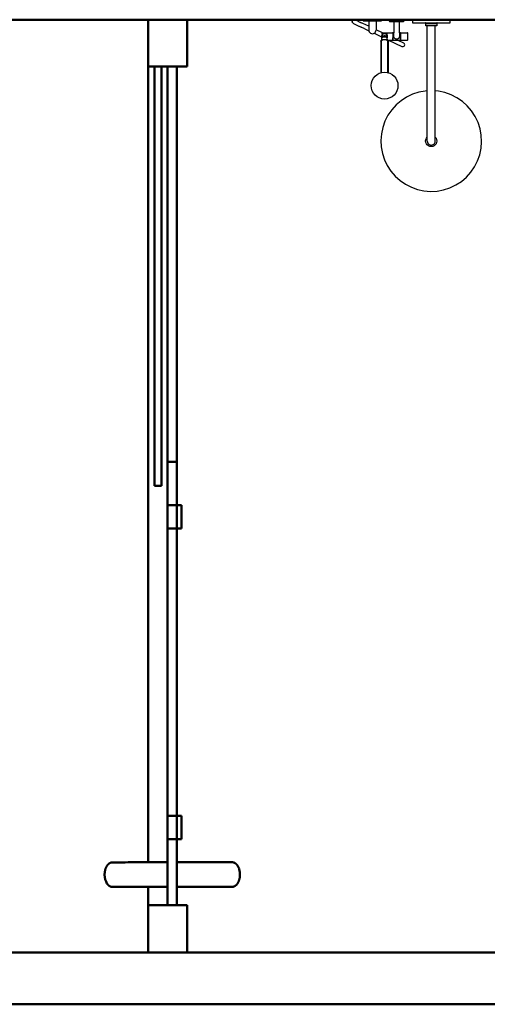
# Model space of a CAD drawing. Units: inches. Extents: x 64 to 1167, y 117 to 939.
# Tile 18 of 56: x 248 to 284, y 781 to 857. Entities that reach past the tile are written whole.
import ezdxf

# ---------------------------------------------------------------- set-up
doc = ezdxf.new("R2010")
doc.units = ezdxf.units.IN
doc.header["$MEASUREMENT"] = 0
doc.layers.add('A-FLOR-FIXT', color=8, linetype='Continuous', lineweight=18)
doc.layers.add('A-WALL', color=7, linetype='Continuous', lineweight=50)
doc.layers.add('Edges', color=7, linetype='Continuous')

# ---------------------------------------------------------------- blocks, each defined once
blk = doc.blocks.new('Handheld Shower set pl')
at = {"layer": 'Edges'}
for p, q in [((254.9, 328.7), (274.2, 319.6)), ((262, 340.8), (280.2, 332.2)), ((274.2, 319.6), (276.7, 318.4)), ((279.6, 317), (276.7, 318.4)), ((279.6, 317), (281.6, 316)), ((287.6, 328.7), (280.2, 332.2)), ((280.2, 332.2), (282.7, 331)), ((294.8, 309.8), (281.6, 316)), ((308.3, 318.9), (287.6, 328.7)), ((352.8, 340.8), (289.3, 340.8)), ((289.3, 340.8), (289.3, 337.7)), ((289.3, 337.7), (308.4, 337.7)), ((294.8, 309.8), (308.8, 303.2)), ((308.3, 318.9), (308.4, 318.8)), ((308.4, 337.7), (308.4, 318.8)), ((308.4, 337.7), (333.8, 337.7)), ((308.4, 318.8), (308.4, 305.9)), ((333.8, 337.7), (333.8, 306.8)), ((333.8, 337.7), (352.8, 337.7)), ((352.8, 340.8), (352.8, 337.7)), ((379.7, 340.5), (379.7, 336.5)), ((380.1, 340.7), (430.2, 340.7)), ((380.1, 336.2), (430.2, 336.2)), ((381.6, 335.3), (428.8, 335.3)), ((395.6, 335.3), (395.6, 296.4)), ((414.6, 296.4), (414.6, 335.3)), ((430.5, 340.5), (430.5, 336.5)), ((460.1, 340.8), (460.1, 330.7)), ((591.7, 340.8), (460.1, 340.8)), ((460.1, 330.7), (505.5, 330.7)), ((505.7, 330.7), (505.5, 330.7)), ((505.9, 330.6), (505.7, 330.7)), ((505.7, 330.7), (545.6, 330.7)), ((506.1, 330.5), (505.9, 330.6)), ((506.3, 330.4), (506.1, 330.5)), ((506.5, 330.3), (506.3, 330.4)), ((506.6, 330.1), (506.5, 330.3)), ((506.7, 329.9), (506.6, 330.1)), ((506.8, 329.7), (506.7, 329.9)), ((506.9, 329.5), (506.8, 329.7)), ((506.9, 329.3), (506.9, 329.5)), ((506.9, 329.1), (506.9, 329.3)), ((544.4, 329.1), (506.9, 329.1)), ((506.9, 320.4), (506.9, 328.9)), ((506.9, 328.9), (544.4, 328.9)), ((511.4, 320.4), (506.9, 320.4)), ((511.4, 94.2), (511.4, 320.4)), ((539.4, 320.4), (511.4, 320.4)), ((539.4, 94.2), (539.4, 320.4)), ((544.4, 320.4), (539.4, 320.4)), ((544.5, 329.5), (544.4, 329.3)), ((544.4, 329.3), (544.4, 329.1)), ((544.4, 328.9), (544.4, 320.4)), ((544.6, 329.9), (544.5, 329.7)), ((544.5, 329.7), (544.5, 329.5)), ((544.7, 330.1), (544.6, 329.9)), ((544.9, 330.3), (544.7, 330.1)), ((545, 330.4), (544.9, 330.3)), ((545.2, 330.5), (545, 330.4)), ((545.4, 330.6), (545.2, 330.5)), ((545.6, 330.7), (545.4, 330.6)), ((545.8, 330.7), (545.6, 330.7)), ((545.8, 330.7), (591.7, 330.7)), ((591.7, 330.7), (591.7, 340.8)), ((308.4, 305.9), (308.8, 303.2)), ((308.8, 303.2), (308.8, 302.6)), ((308.8, 302.6), (310.1, 299.6)), ((310.1, 299.6), (312.1, 296.9)), ((312.1, 296.9), (314.7, 294.9)), ((314.7, 294.9), (317.8, 293.7)), ((317.8, 293.7), (321.1, 293.2)), ((321.1, 293.2), (324.4, 293.7)), ((324.4, 293.7), (326.7, 294.6)), ((326.7, 294.6), (327.4, 294.9)), ((326.7, 294.6), (352.9, 282.2)), ((327.4, 294.9), (330.1, 296.9)), ((330.1, 296.9), (332.1, 299.6)), ((332.1, 299.6), (333.4, 302.6)), ((333.4, 302.6), (333.8, 305.9)), ((333.8, 306.8), (333.8, 305.9)), ((355.7, 296.4), (333.8, 306.8)), ((352.9, 285.6), (352.8, 284.3)), ((352.8, 284.3), (352.8, 283)), ((352.8, 283), (352.9, 282.2)), ((353.2, 286.9), (352.9, 285.6)), ((352.9, 282.2), (352.9, 281.8)), ((352.9, 281.8), (353.2, 280.5)), ((353.7, 288.1), (353.2, 286.9)), ((353.2, 280.5), (353.6, 279.7)), ((353.5, 296.4), (355.7, 296.4)), ((353.5, 296.4), (353.5, 293.2)), ((353.5, 293.2), (359.1, 293.2)), ((353.5, 274.2), (353.6, 278.1)), ((353.5, 271.2), (353.5, 274.2)), ((353.5, 274.2), (353.6, 274.2)), ((353.7, 285.5), (353.6, 284.3)), ((353.6, 283), (353.6, 284.3)), ((353.6, 283), (353.6, 282.5)), ((353.6, 282.5), (353.9, 283)), ((353.6, 283), (353.6, 281.9)), ((353.6, 282.1), (353.6, 282.5)), ((353.6, 281.9), (353.6, 282.1)), ((353.6, 282.1), (353.6, 281.3)), ((353.6, 281.3), (353.6, 281.9)), ((353.6, 279.7), (353.6, 281.9)), ((353.6, 279.7), (353.6, 279.5)), ((353.6, 278.6), (353.6, 279.7)), ((353.7, 279.1), (353.6, 278.6)), ((353.6, 278.6), (353.6, 278.1)), ((353.6, 278.1), (353.6, 277.9)), ((354.3, 289.2), (353.7, 288.1)), ((354, 286.6), (353.7, 285.5)), ((353.7, 279.1), (354, 279.6)), ((353.9, 283), (354.2, 283.5)), ((354.4, 287.8), (354, 286.6)), ((354, 279.6), (354.4, 280.1)), ((354.2, 283.5), (354.7, 284)), ((355.1, 290.3), (354.3, 289.2)), ((355, 288.8), (354.4, 287.8)), ((354.4, 280.1), (355, 280.5)), ((354.7, 284), (355.4, 284.5)), ((355.7, 289.8), (355, 288.8)), ((355, 280.5), (355.7, 280.9)), ((356, 291.2), (355.1, 290.3)), ((355.4, 284.5), (356.1, 284.9)), ((355.7, 296.4), (391.2, 296.4)), ((356.5, 290.6), (355.7, 289.8)), ((355.7, 280.9), (356.5, 281.3)), ((357, 292), (356, 291.2)), ((356.1, 284.9), (357, 285.3)), ((357.5, 291.4), (356.5, 290.6)), ((356.5, 281.3), (357.5, 281.6)), ((358.1, 292.7), (357, 292)), ((357, 285.3), (358, 285.7)), ((358.5, 292), (357.5, 291.4)), ((357.5, 281.6), (358.5, 281.9)), ((358, 285.7), (359, 285.9)), ((359.1, 293.2), (358.1, 292.7)), ((359.6, 292.6), (358.5, 292)), ((358.5, 281.9), (359.6, 282.1)), ((359, 285.9), (360.1, 286.2)), ((359.3, 293.3), (359.1, 293.2)), ((360.5, 293.7), (359.3, 293.3)), ((360.7, 292.9), (359.6, 292.6)), ((359.6, 282.1), (360.7, 282.3)), ((360.1, 286.2), (361.3, 286.3)), ((361.8, 293.9), (360.5, 293.7)), ((361.9, 293.1), (360.7, 292.9)), ((360.7, 282.3), (361.9, 282.4)), ((361.3, 286.3), (362.5, 286.4)), ((363.1, 294), (361.8, 293.9)), ((363.1, 293.2), (361.9, 293.1)), ((361.9, 282.4), (363.1, 282.4)), ((362.5, 286.4), (363.7, 286.4)), ((363.1, 292.9), (363.1, 297.1)), ((364.4, 293.9), (363.1, 294)), ((364.3, 293.1), (363.1, 293.2)), ((364.3, 282.4), (363.1, 282.4)), ((363.7, 286.4), (364.8, 286.3)), ((365.4, 292.9), (364.3, 293.1)), ((364.3, 282.4), (365.4, 282.3)), ((365.6, 293.7), (364.4, 293.9)), ((364.8, 286.3), (366, 286.2)), ((366.6, 292.6), (365.4, 292.9)), ((365.4, 282.3), (366.6, 282.1)), ((366.9, 293.3), (365.6, 293.7)), ((366, 286.2), (367.1, 285.9)), ((367.6, 292), (366.6, 292.6)), ((366.6, 282.1), (367.6, 281.9)), ((367, 293.2), (366.9, 293.3)), ((368, 292.7), (367, 293.2)), ((367, 293.2), (372.6, 293.2)), ((367.1, 285.9), (368.2, 285.7)), ((368.7, 291.4), (367.6, 292)), ((367.6, 281.9), (368.7, 281.6)), ((369.1, 292), (368, 292.7)), ((368.2, 285.7), (369.1, 285.3)), ((369.6, 290.6), (368.7, 291.4)), ((368.7, 281.6), (369.6, 281.3)), ((370.1, 291.2), (369.1, 292)), ((369.1, 285.3), (370, 284.9)), ((370.4, 289.8), (369.6, 290.6)), ((369.6, 281.3), (370.4, 280.9)), ((370, 284.9), (370.7, 284.5)), ((371, 290.3), (370.1, 291.2)), ((371.1, 288.8), (370.4, 289.8)), ((370.4, 280.9), (371.1, 280.5)), ((370.7, 284.5), (371.4, 284)), ((371.8, 289.2), (371, 290.3)), ((371.7, 287.8), (371.1, 288.8)), ((371.1, 280.5), (371.7, 280.1)), ((371.4, 284), (371.9, 283.5)), ((372.1, 286.6), (371.7, 287.8)), ((371.7, 280.1), (372.1, 279.6)), ((372.2, 288.5), (371.8, 289.2)), ((371.9, 283.5), (372.3, 283)), ((372.4, 285.5), (372.1, 286.6)), ((372.1, 279.6), (372.4, 279.2)), ((372.6, 288.3), (372.2, 288.5)), ((372.4, 288.1), (372.2, 288.5)), ((372.3, 283), (372.5, 282.5)), ((372.3, 281.3), (372.4, 281.9)), ((372.3, 280.7), (372.5, 281.3)), ((372.3, 277.4), (372.4, 277.6)), ((372.3, 274.2), (372.6, 274.2)), ((372.6, 287.7), (372.4, 288.1)), ((372.6, 284.3), (372.4, 285.5)), ((372.4, 281.9), (372.5, 282.3)), ((372.4, 279.3), (372.6, 279.7)), ((372.4, 279.2), (372.4, 279.3)), ((372.4, 279.1), (372.4, 279.2)), ((372.6, 278.6), (372.4, 279.1)), ((372.4, 277.6), (372.6, 278.1)), ((372.5, 282.5), (372.6, 283)), ((372.5, 282.5), (372.5, 282.3)), ((372.5, 282.1), (372.5, 282.3)), ((372.5, 282.1), (372.6, 281.9)), ((372.5, 282.1), (372.5, 281.3)), ((372.6, 281.9), (372.5, 281.3)), ((372.6, 288.3), (372.6, 293.2)), ((372.6, 288.3), (372.6, 287.7)), ((372.9, 286.9), (372.6, 287.7)), ((372.6, 283), (372.6, 284.3)), ((372.6, 283), (372.6, 281.9)), ((372.6, 281.9), (372.6, 279.7)), ((372.6, 279.7), (372.9, 280.5)), ((372.6, 279.7), (372.6, 278.6)), ((372.6, 278.1), (372.6, 278.6)), ((372.6, 274.2), (372.6, 278.1)), ((372.6, 274.2), (372.6, 271)), ((373.2, 285.6), (372.9, 286.9)), ((372.9, 280.5), (373.2, 281.8)), ((373.4, 284.3), (373.2, 285.6)), ((373.2, 281.8), (373.4, 283)), ((373.4, 283), (373.4, 284.3)), ((391.6, 296), (391.6, 271.4)), ((392, 295.6), (391.6, 295.6)), ((392, 295.6), (392, 279.3)), ((392, 295.6), (392, 279.1)), ((392, 279.3), (392, 279.1)), ((392, 279.3), (392, 279.1)), ((392, 279.1), (392, 278)), ((392, 279.1), (392, 278)), ((392, 279.1), (392, 279.1)), ((392, 279.1), (392, 279.1)), ((392, 271.8), (392, 279.1)), ((392, 271.8), (392, 278)), ((393.2, 296.4), (395.6, 296.4)), ((395.6, 283.7), (395.6, 296.4)), ((395.7, 282.5), (395.6, 283.7)), ((395.9, 281.3), (395.7, 282.5)), ((396.3, 280.2), (395.9, 281.3)), ((396.8, 279.1), (396.3, 280.2)), ((397.4, 278.1), (396.8, 279.1)), ((398.2, 277.2), (397.4, 278.1)), ((399, 276.4), (398.2, 277.2)), ((400, 275.7), (399, 276.4)), ((401.1, 275.1), (400, 275.7)), ((402.2, 274.6), (401.1, 275.1)), ((403.3, 274.3), (402.2, 274.6)), ((404.5, 274.2), (403.3, 274.3)), ((405.7, 274.2), (404.5, 274.2)), ((406.9, 274.3), (405.7, 274.2)), ((408.1, 274.6), (406.9, 274.3)), ((409.2, 275.1), (408.1, 274.6)), ((410.2, 275.7), (409.2, 275.1)), ((411.2, 276.4), (410.2, 275.7)), ((412.1, 277.2), (411.2, 276.4)), ((412.8, 278.1), (412.1, 277.2)), ((413.5, 279.1), (412.8, 278.1)), ((414, 280.2), (413.5, 279.1)), ((414.3, 281.3), (414, 280.2)), ((414.6, 282.5), (414.3, 281.3)), ((414.6, 296.4), (417, 296.4)), ((414.6, 296.4), (414.6, 283.7)), ((414.6, 283.7), (414.6, 282.5)), ((418.2, 295.6), (418.2, 279.3)), ((418.2, 295.6), (418.2, 279.1)), ((418.2, 295.6), (418.6, 295.6)), ((418.2, 271.8), (418.2, 279.1)), ((418.2, 271.8), (418.2, 278)), ((418.6, 296), (418.6, 271.4)), ((419, 296.4), (443.2, 296.4)), ((443.9, 272), (443.9, 295.4)), ((350.4, 266.9), (350.5, 267.6)), ((350.4, 266.9), (350.4, 157.5)), ((350.5, 267.6), (350.8, 268.3)), ((350.8, 268.3), (351.3, 269)), ((351.3, 269), (351.9, 269.7)), ((351.9, 269.7), (352.8, 270.3)), ((352.8, 270.3), (353.1, 270.5)), ((353.3, 270.7), (353.1, 270.6)), ((353.1, 270.5), (353.1, 270.6)), ((353.1, 263.2), (353.1, 270.5)), ((353.1, 158.2), (353.1, 263.2)), ((353.4, 270.7), (353.3, 270.7)), ((353.5, 270.7), (353.4, 270.7)), ((353.5, 271.2), (353.5, 271)), ((353.6, 271), (353.5, 271.2)), ((353.5, 271), (353.6, 271)), ((353.6, 270.8), (353.5, 270.7)), ((353.6, 270.8), (353.6, 271)), ((353.6, 270.8), (353.8, 270.9)), ((353.8, 270.9), (353.6, 270.8)), ((353.6, 270.8), (353.6, 270.8)), ((353.6, 270.8), (353.6, 270.8)), ((353.8, 270.8), (353.9, 270.9)), ((353.8, 270.9), (353.8, 270.8)), ((353.9, 270.9), (354.1, 270.9)), ((354.1, 270.9), (354.2, 271)), ((354.2, 271), (354.4, 271)), ((354.4, 271), (354.5, 271)), ((354.5, 271), (354.7, 271.1)), ((354.7, 271.1), (354.9, 271.1)), ((354.9, 271.1), (355.1, 271.1)), ((355.1, 271.1), (355.2, 271.2)), ((355.2, 271.2), (355.4, 271.2)), ((355.4, 271.2), (355.6, 271.2)), ((355.6, 271.2), (355.8, 271.2)), ((355.8, 271.2), (355.9, 271.2)), ((355.9, 271.2), (356.1, 271.3)), ((356.1, 271.3), (356.3, 271.3)), ((356.3, 271.3), (356.4, 271.3)), ((356.6, 271.3), (356.4, 271.3)), ((356.7, 271.3), (356.6, 271.3)), ((356.9, 271.3), (356.7, 271.3)), ((369.2, 271.3), (356.9, 271.3)), ((369.4, 271.3), (369.2, 271.3)), ((369.5, 271.3), (369.4, 271.3)), ((369.5, 271.3), (369.7, 271.3)), ((369.7, 271.3), (369.8, 271.3)), ((369.8, 271.3), (370, 271.3)), ((370, 271.3), (370.2, 271.2)), ((370.2, 271.2), (370.4, 271.2)), ((370.4, 271.2), (370.5, 271.2)), ((370.5, 271.2), (370.7, 271.2)), ((370.7, 271.2), (370.9, 271.2)), ((370.9, 271.2), (371.1, 271.1)), ((371.1, 271.1), (371.2, 271.1)), ((371.2, 271.1), (371.4, 271.1)), ((371.4, 271.1), (371.6, 271)), ((371.6, 271), (371.7, 271)), ((371.7, 271), (371.9, 271)), ((371.9, 271), (372.1, 270.9)), ((372.1, 270.9), (372.2, 270.9)), ((372.2, 270.9), (372.3, 270.8)), ((372.3, 271), (372.6, 271)), ((372.3, 270.9), (372.3, 270.8)), ((372.3, 270.9), (372.5, 270.8)), ((372.3, 270.8), (372.4, 270.8)), ((372.4, 270.8), (372.5, 270.8)), ((372.5, 270.8), (372.5, 270.8)), ((372.5, 270.8), (372.6, 270.8)), ((372.6, 271), (376.4, 271)), ((372.6, 271), (372.6, 270.8)), ((372.6, 270.8), (372.6, 270.7)), ((372.6, 270.7), (372.7, 270.7)), ((372.7, 270.7), (372.9, 270.7)), ((372.7, 270.7), (372.9, 270.6)), ((372.7, 270.7), (372.7, 270.7)), ((372.9, 270.7), (373, 270.6)), ((372.9, 270.7), (372.9, 270.6)), ((372.9, 270.6), (373, 270.5)), ((373, 270.6), (373, 270.5)), ((373, 270.5), (373, 158.3)), ((373, 270.5), (373.3, 270.3)), ((373.3, 270.3), (374.2, 269.7)), ((374.2, 269.7), (374.9, 269)), ((374.9, 269), (375.4, 268.3)), ((375.4, 268.3), (375.7, 267.6)), ((375.7, 267.6), (375.8, 266.9)), ((375.8, 266.9), (375.8, 157.6)), ((376.4, 271), (391.2, 271)), ((376.4, 271), (423.4, 248.7)), ((392, 271.8), (391.6, 271.8)), ((392, 271.8), (392, 271.8)), ((392, 271.8), (392.4, 271.8)), ((392, 271.8), (392.4, 271.8)), ((392.4, 271.8), (392.4, 271.8)), ((392.4, 271.7), (392.4, 271.8)), ((392.4, 271.6), (392.4, 271.7)), ((392.4, 271.7), (392.4, 271.7)), ((392.5, 271.6), (392.4, 271.6)), ((392.5, 271.5), (392.5, 271.6)), ((392.5, 271.5), (392.5, 271.5)), ((392.5, 271.4), (392.5, 271.5)), ((392.5, 271.4), (392.5, 271.4)), ((392.6, 271.3), (392.5, 271.4)), ((392.7, 271.2), (392.6, 271.3)), ((392.6, 271.3), (392.6, 271.3)), ((392.6, 271.3), (392.6, 271.3)), ((392.7, 271.2), (392.7, 271.2)), ((392.8, 271.2), (392.7, 271.2)), ((392.8, 271.1), (392.8, 271.2)), ((392.9, 271.1), (392.8, 271.1)), ((393, 271.1), (392.9, 271.1)), ((392.9, 271.1), (392.9, 271.1)), ((392.9, 271.1), (392.9, 271.1)), ((393, 271), (393, 271.1)), ((393, 271), (393.1, 271)), ((393.1, 271), (393.2, 271)), ((393.2, 271), (393.2, 271)), ((393.2, 271), (409, 271)), ((409, 271), (417, 271)), ((409, 271), (429.4, 261.4)), ((417.1, 271), (417, 271)), ((417.1, 271), (417.1, 271)), ((417.2, 271), (417.1, 271)), ((417.2, 271), (417.2, 271.1)), ((417.2, 271.1), (417.3, 271.1)), ((417.3, 271.1), (417.4, 271.1)), ((417.3, 271.1), (417.3, 271.1)), ((417.4, 271.1), (417.6, 271.3)), ((417.6, 271.3), (417.7, 271.4)), ((417.6, 271.3), (417.6, 271.3)), ((417.6, 271.3), (417.6, 271.3)), ((417.7, 271.5), (417.8, 271.6)), ((417.7, 271.5), (417.7, 271.5)), ((417.7, 271.4), (417.7, 271.5)), ((417.7, 271.4), (417.7, 271.4)), ((417.8, 271.8), (417.8, 271.8)), ((417.8, 271.7), (417.8, 271.8)), ((418.2, 271.8), (417.8, 271.8)), ((418.2, 271.8), (417.8, 271.8)), ((417.8, 271.6), (417.8, 271.7)), ((417.8, 271.7), (417.8, 271.7)), ((417.8, 271.6), (417.8, 271.6)), ((418.2, 271.8), (418.2, 271.8)), ((418.2, 271.8), (418.6, 271.8)), ((419, 271), (443.2, 271)), ((423.4, 248.7), (427.7, 248.2)), ((427.7, 248.2), (431, 249.9)), ((432.5, 258.3), (429.4, 261.4)), ((431, 249.9), (432.7, 252.1)), ((433.3, 254.7), (432.5, 258.3)), ((432.7, 252.1), (433.3, 254.7)), ((440, 72.8), (420.8, 60.4)), ((460.6, 82.7), (440, 72.8)), ((482.4, 89.7), (460.6, 82.7)), ((504.9, 93.9), (482.4, 89.7)), ((511.4, 94.2), (504.9, 93.9)), ((511.4, -66.4), (511.4, 94.2)), ((550.6, 93.3), (539.4, 94.2)), ((539.4, -66.4), (539.4, 94.2)), ((573, 88.5), (550.6, 93.3)), ((594.6, 80.9), (573, 88.5)), ((614.9, 70.5), (594.6, 80.9)), ((633.8, 57.5), (614.9, 70.5)), ((403.4, 45.5), (388, 28.5)), ((420.8, 60.4), (403.4, 45.5)), ((650.8, 42.2), (633.8, 57.5)), ((665.7, 24.8), (650.8, 42.2)), ((375.1, 9.6), (364.7, -10.8)), ((388, 28.5), (375.1, 9.6)), ((678.1, 5.6), (665.7, 24.8)), ((688, -15.1), (678.1, 5.6)), ((357, -32.3), (352.2, -54.7)), ((364.7, -10.8), (357, -32.3)), ((695, -36.9), (688, -15.1)), ((352.2, -54.7), (350.4, -77.5)), ((508.6, -70.1), (511.4, -66.4)), ((511.4, -79.8), (511.4, -66.4)), ((539.4, -66.4), (542.2, -70.1)), ((539.4, -79.8), (539.4, -66.4)), ((699.2, -59.4), (695, -36.9)), ((700.4, -82.3), (699.2, -59.4)), ((350.4, -77.5), (351.6, -100.4)), ((351.6, -100.4), (355.8, -122.9)), ((506, -79.8), (506.7, -74.8)), ((506.7, -84.8), (506, -79.8)), ((506.7, -74.8), (508.6, -70.1)), ((508.6, -89.5), (506.7, -84.8)), ((511.7, -93.5), (508.6, -89.5)), ((511.4, -79.8), (511.9, -83.4)), ((515.7, -96.6), (511.7, -93.5)), ((511.9, -83.4), (513.3, -86.8)), ((513.3, -86.8), (515.5, -89.7)), ((515.5, -89.7), (518.4, -91.9)), ((520.4, -98.5), (515.7, -96.6)), ((518.4, -91.9), (521.8, -93.3)), ((525.4, -99.2), (520.4, -98.5)), ((521.8, -93.3), (525.4, -93.8)), ((525.4, -93.8), (529, -93.3)), ((530.4, -98.5), (525.4, -99.2)), ((529, -93.3), (532.4, -91.9)), ((535.1, -96.6), (530.4, -98.5)), ((532.4, -91.9), (535.3, -89.7)), ((539.1, -93.5), (535.1, -96.6)), ((535.3, -89.7), (537.5, -86.8)), ((537.5, -86.8), (538.9, -83.4)), ((538.9, -83.4), (539.4, -79.8)), ((542.2, -89.5), (539.1, -93.5)), ((542.2, -70.1), (544.1, -74.8)), ((544.1, -84.8), (542.2, -89.5)), ((544.1, -74.8), (544.8, -79.8)), ((544.8, -79.8), (544.1, -84.8)), ((698.6, -105.1), (700.4, -82.3)), ((355.8, -122.9), (362.9, -144.7)), ((686.2, -149), (693.8, -127.5)), ((693.8, -127.5), (698.6, -105.1)), ((362.9, -144.7), (372.7, -165.3)), ((372.7, -165.3), (385.2, -184.6)), ((662.8, -188.3), (675.8, -169.4)), ((675.8, -169.4), (686.2, -149)), ((385.2, -184.6), (400, -202)), ((400, -202), (417, -217.3)), ((630.1, -220.2), (647.5, -205.3)), ((647.5, -205.3), (662.8, -188.3)), ((417, -217.3), (435.9, -230.3)), ((435.9, -230.3), (456.3, -240.7)), ((590.2, -242.5), (610.9, -232.6)), ((610.9, -232.6), (630.1, -220.2)), ((456.3, -240.7), (477.9, -248.3)), ((477.9, -248.3), (500.2, -253.1)), ((500.2, -253.1), (523.1, -254.9)), ((523.1, -254.9), (545.9, -253.7)), ((545.9, -253.7), (568.4, -249.5)), ((568.4, -249.5), (590.2, -242.5))]:
    blk.add_line(p, q, dxfattribs=at)
blk.add_lwpolyline([(254.9, 328.7), (253.9, 329.7), (253.1, 330.5), (252.5, 331), (252.2, 331.4), (251.9, 331.7), (251.8, 332), (251.7, 332.2), (251.6, 332.4), (251.6, 332.6), (251.5, 332.9), (251.4, 333.3), (251.4, 333.6), (251.3, 334), (251.3, 334.4), (251.2, 334.8), (251.2, 335.2), (251.2, 335.6), (251.2, 336), (251.3, 336.3), (251.4, 336.7), (251.4, 337), (251.6, 337.3), (251.7, 337.6), (251.8, 337.9), (252, 338.2), (252.1, 338.5), (252.3, 338.8), (252.5, 339.1), (252.7, 339.4), (253, 339.6), (253.3, 339.9), (253.6, 340.1), (253.9, 340.4), (254.2, 340.6), (254.5, 340.8), (254.9, 341), (255.2, 341.2), (255.5, 341.3), (255.8, 341.5), (256, 341.6), (256.2, 341.7), (256.4, 341.8), (256.5, 341.8), (256.6, 341.8), (256.8, 341.8), (257, 341.8), (257.3, 341.8), (257.7, 341.7), (258.1, 341.7), (258.6, 341.6), (259.2, 341.5), (259.8, 341.4), (260.4, 341.3), (261, 341.2), (261.6, 341), (262, 340.8)], dxfattribs=at)
blk.add_circle((363.2, 112.7), 46.6, dxfattribs=at)
for centre, radius, start, end in [((380, 340.3), 0.344, 86.4523, 162.0345), ((380, 336.6), 0.344, 197.9655, 273.5477), ((381.6, 336.4), 1.16, 189.8715, 268.521), ((428.8, 336.4), 1.16, 271.479, 350.1285), ((430.2, 340.3), 0.344, 17.9655, 93.5477), ((430.2, 336.6), 0.344, 266.4523, 342.0345), ((391.1, 295.9), 0.512, 11.477, 75.5526), ((393.6, 294.5), 1.97, 102.3058, 144.97), ((416.6, 294.5), 1.97, 35.03, 77.6942), ((419.1, 295.9), 0.512, 104.4474, 168.523), ((442.8, 295.4), 1.08, 2.6678, 69.8908), ((391.1, 271.5), 0.512, 284.4474, 348.523), ((419.1, 271.5), 0.512, 191.477, 255.5526), ((442.8, 272), 1.08, 290.1092, 357.3322)]:
    blk.add_arc(centre, radius, start, end, dxfattribs=at)

msp = doc.modelspace()

# ---------------------------------------------------------------- linework, layer by layer
at = {"layer": 'A-WALL'}
for p, q in [((297.107, 857.2), (183.107, 857.2)), ((261.006, 857.2), (258.008, 857.2)), ((258.008, 857.2), (258.008, 853.603)), ((261.006, 857.2), (261.006, 853.603)), ((258.008, 853.603), (258.008, 792.162)), ((258.488, 853.603), (258.008, 853.603)), ((259.027, 853.603), (258.488, 853.603)), ((258.488, 853.603), (258.488, 821.23)), ((259.507, 853.603), (259.027, 853.603)), ((259.027, 853.603), (259.027, 821.23)), ((259.507, 823.088), (259.507, 853.603)), ((260.226, 853.603), (259.507, 853.603)), ((261.006, 853.603), (260.226, 853.603)), ((260.226, 823.088), (260.226, 853.603)), ((260.226, 823.088), (259.507, 823.088)), ((259.507, 819.731), (259.507, 823.088)), ((260.226, 819.731), (260.226, 823.088)), ((258.488, 821.23), (259.027, 821.23)), ((260.226, 819.731), (259.507, 819.731)), ((259.507, 817.932), (259.507, 819.731)), ((260.226, 817.932), (260.226, 819.731)), ((260.226, 819.731), (260.586, 819.731)), ((260.586, 817.932), (260.586, 819.731)), ((259.507, 795.751), (259.507, 817.932)), ((260.226, 817.932), (259.507, 817.932)), ((260.226, 795.751), (260.226, 817.932)), ((260.226, 817.932), (260.586, 817.932)), ((260.226, 795.751), (259.507, 795.751)), ((259.507, 793.952), (259.507, 795.751)), ((260.226, 795.751), (260.226, 793.952)), ((260.226, 795.751), (260.586, 795.751)), ((260.586, 795.751), (260.586, 793.952)), ((260.226, 793.952), (259.507, 793.952)), ((259.507, 793.952), (259.507, 792.162)), ((260.226, 792.17), (260.226, 793.952)), ((260.226, 793.952), (260.586, 793.952)), ((255.149, 792.145), (255.141, 792.143)), ((255.157, 792.147), (255.149, 792.145)), ((255.165, 792.149), (255.157, 792.147)), ((255.174, 792.151), (255.165, 792.149)), ((255.183, 792.153), (255.174, 792.151)), ((255.191, 792.154), (255.183, 792.153)), ((255.2, 792.156), (255.191, 792.154)), ((255.208, 792.156), (255.2, 792.156)), ((255.217, 792.157), (255.208, 792.156)), ((255.226, 792.157), (255.217, 792.157)), ((255.234, 792.158), (255.226, 792.157)), ((255.244, 792.158), (255.234, 792.158)), ((255.253, 792.158), (255.244, 792.158)), ((255.263, 792.158), (255.253, 792.158)), ((255.305, 792.158), (255.263, 792.158)), ((256.227, 792.158), (255.305, 792.158)), ((256.462, 792.162), (256.227, 792.158)), ((258.008, 792.162), (256.462, 792.162)), ((259.507, 792.162), (258.008, 792.162)), ((259.507, 792.162), (259.507, 791.392)), ((260.226, 792.17), (263.272, 792.17)), ((260.226, 792.17), (260.226, 791.392)), ((263.272, 792.17), (263.506, 792.166)), ((264.429, 792.166), (263.506, 792.166)), ((264.47, 792.166), (264.429, 792.166)), ((264.47, 792.166), (264.498, 792.166)), ((264.541, 792.166), (264.498, 792.166)), ((264.541, 792.166), (264.566, 792.159)), ((264.566, 792.159), (264.586, 792.153)), ((264.586, 792.153), (264.602, 792.148)), ((264.602, 792.148), (264.615, 792.145)), ((254.653, 791.394), (254.649, 791.364)), ((254.657, 791.424), (254.653, 791.394)), ((254.662, 791.454), (254.657, 791.424)), ((254.667, 791.483), (254.662, 791.454)), ((254.673, 791.513), (254.667, 791.483)), ((254.68, 791.542), (254.673, 791.513)), ((254.687, 791.57), (254.68, 791.542)), ((254.695, 791.599), (254.687, 791.57)), ((254.703, 791.626), (254.695, 791.599)), ((254.712, 791.654), (254.703, 791.626)), ((254.722, 791.681), (254.712, 791.654)), ((254.732, 791.707), (254.722, 791.681)), ((254.743, 791.733), (254.732, 791.707)), ((254.753, 791.758), (254.743, 791.733)), ((254.765, 791.782), (254.753, 791.758)), ((254.776, 791.805), (254.765, 791.782)), ((254.787, 791.826), (254.776, 791.805)), ((254.798, 791.846), (254.787, 791.826)), ((254.808, 791.865), (254.798, 791.846)), ((254.819, 791.882), (254.808, 791.865)), ((254.828, 791.897), (254.819, 791.882)), ((254.838, 791.91), (254.828, 791.897)), ((254.846, 791.923), (254.838, 791.91)), ((254.854, 791.933), (254.846, 791.923)), ((254.861, 791.942), (254.854, 791.933)), ((254.867, 791.95), (254.861, 791.942)), ((254.873, 791.957), (254.867, 791.95)), ((254.877, 791.962), (254.873, 791.957)), ((254.881, 791.967), (254.877, 791.962)), ((254.884, 791.97), (254.881, 791.967)), ((254.887, 791.974), (254.884, 791.97)), ((254.89, 791.977), (254.887, 791.974)), ((254.893, 791.98), (254.89, 791.977)), ((254.895, 791.983), (254.893, 791.98)), ((254.899, 791.987), (254.895, 791.983)), ((254.902, 791.991), (254.899, 791.987)), ((254.907, 791.996), (254.902, 791.991)), ((254.911, 792.001), (254.907, 791.996)), ((254.916, 792.007), (254.911, 792.001)), ((254.921, 792.013), (254.916, 792.007)), ((254.926, 792.018), (254.921, 792.013)), ((254.932, 792.024), (254.926, 792.018)), ((254.937, 792.029), (254.932, 792.024)), ((254.941, 792.033), (254.937, 792.029)), ((254.946, 792.037), (254.941, 792.033)), ((254.95, 792.041), (254.946, 792.037)), ((254.954, 792.044), (254.95, 792.041)), ((254.958, 792.047), (254.954, 792.044)), ((254.961, 792.049), (254.958, 792.047)), ((254.964, 792.051), (254.961, 792.049)), ((254.967, 792.053), (254.964, 792.051)), ((254.969, 792.055), (254.967, 792.053)), ((254.971, 792.056), (254.969, 792.055)), ((254.973, 792.058), (254.971, 792.056)), ((254.975, 792.059), (254.973, 792.058)), ((254.978, 792.061), (254.975, 792.059)), ((254.98, 792.062), (254.978, 792.061)), ((254.983, 792.064), (254.98, 792.062)), ((254.987, 792.067), (254.983, 792.064)), ((254.991, 792.07), (254.987, 792.067)), ((254.996, 792.073), (254.991, 792.07)), ((255.002, 792.076), (254.996, 792.073)), ((255.008, 792.08), (255.002, 792.076)), ((255.014, 792.084), (255.008, 792.08)), ((255.021, 792.088), (255.014, 792.084)), ((255.027, 792.092), (255.021, 792.088)), ((255.034, 792.096), (255.027, 792.092)), ((255.041, 792.101), (255.034, 792.096)), ((255.047, 792.105), (255.041, 792.101)), ((255.054, 792.109), (255.047, 792.105)), ((255.06, 792.113), (255.054, 792.109)), ((255.066, 792.116), (255.06, 792.113)), ((255.072, 792.119), (255.066, 792.116)), ((255.078, 792.123), (255.072, 792.119)), ((255.083, 792.125), (255.078, 792.123)), ((255.088, 792.128), (255.083, 792.125)), ((255.093, 792.129), (255.088, 792.128)), ((255.098, 792.131), (255.093, 792.129)), ((255.103, 792.133), (255.098, 792.131)), ((255.108, 792.134), (255.103, 792.133)), ((255.114, 792.136), (255.108, 792.134)), ((255.12, 792.137), (255.114, 792.136)), ((255.126, 792.139), (255.12, 792.137)), ((255.133, 792.141), (255.126, 792.139)), ((255.141, 792.143), (255.133, 792.141)), ((259.507, 791.295), (259.507, 791.392)), ((260.226, 791.392), (260.226, 791.295)), ((264.615, 792.145), (264.626, 792.142)), ((264.626, 792.142), (264.634, 792.139)), ((264.634, 792.139), (264.641, 792.137)), ((264.641, 792.137), (264.648, 792.134)), ((264.648, 792.134), (264.654, 792.131)), ((264.654, 792.131), (264.66, 792.128)), ((264.66, 792.128), (264.667, 792.124)), ((264.667, 792.124), (264.673, 792.121)), ((264.673, 792.121), (264.68, 792.117)), ((264.68, 792.117), (264.686, 792.113)), ((264.686, 792.113), (264.693, 792.109)), ((264.693, 792.109), (264.7, 792.105)), ((264.7, 792.105), (264.706, 792.1)), ((264.706, 792.1), (264.713, 792.096)), ((264.713, 792.096), (264.72, 792.092)), ((264.72, 792.092), (264.727, 792.088)), ((264.727, 792.088), (264.733, 792.084)), ((264.733, 792.084), (264.74, 792.079)), ((264.74, 792.079), (264.746, 792.075)), ((264.746, 792.075), (264.752, 792.071)), ((264.752, 792.071), (264.758, 792.068)), ((264.758, 792.068), (264.764, 792.064)), ((264.764, 792.064), (264.77, 792.06)), ((264.77, 792.06), (264.775, 792.056)), ((264.775, 792.056), (264.78, 792.052)), ((264.78, 792.052), (264.786, 792.047)), ((264.786, 792.047), (264.792, 792.042)), ((264.792, 792.042), (264.797, 792.036)), ((264.797, 792.036), (264.803, 792.03)), ((264.803, 792.03), (264.81, 792.024)), ((264.81, 792.024), (264.816, 792.017)), ((264.816, 792.017), (264.822, 792.011)), ((264.822, 792.011), (264.828, 792.004)), ((264.828, 792.004), (264.833, 791.998)), ((264.833, 791.998), (264.838, 791.992)), ((264.838, 791.992), (264.843, 791.987)), ((264.843, 791.987), (264.846, 791.982)), ((264.846, 791.982), (264.85, 791.978)), ((264.85, 791.978), (264.853, 791.974)), ((264.853, 791.974), (264.856, 791.97)), ((264.856, 791.97), (264.859, 791.966)), ((264.859, 791.966), (264.863, 791.961)), ((264.863, 791.961), (264.868, 791.956)), ((264.868, 791.956), (264.873, 791.949)), ((264.873, 791.949), (264.88, 791.94)), ((264.88, 791.94), (264.889, 791.928)), ((264.889, 791.928), (264.901, 791.911)), ((264.901, 791.911), (264.916, 791.888)), ((264.916, 791.888), (264.934, 791.856)), ((264.934, 791.856), (264.957, 791.814)), ((264.957, 791.814), (264.984, 791.761)), ((264.984, 791.761), (265.018, 791.694)), ((265.018, 791.694), (265.038, 791.613)), ((265.038, 791.613), (265.054, 791.541)), ((265.054, 791.541), (265.067, 791.476)), ((265.067, 791.476), (265.076, 791.419)), ((265.076, 791.419), (265.083, 791.368)), ((254.642, 791.241), (254.641, 791.21)), ((254.641, 791.21), (254.642, 791.179)), ((254.643, 791.272), (254.642, 791.241)), ((254.642, 791.179), (254.643, 791.148)), ((254.644, 791.302), (254.643, 791.272)), ((254.643, 791.148), (254.644, 791.117)), ((254.646, 791.333), (254.644, 791.302)), ((254.644, 791.117), (254.647, 791.085)), ((254.649, 791.364), (254.646, 791.333)), ((254.647, 791.085), (254.651, 791.052)), ((254.651, 791.052), (254.655, 791.019)), ((254.655, 791.019), (254.66, 790.984)), ((254.66, 790.984), (254.667, 790.948)), ((254.667, 790.948), (254.674, 790.91)), ((254.674, 790.91), (254.684, 790.87)), ((254.684, 790.87), (254.696, 790.826)), ((254.696, 790.826), (254.71, 790.779)), ((254.71, 790.779), (254.729, 790.728)), ((254.729, 790.728), (254.752, 790.671)), ((254.752, 790.671), (254.779, 790.607)), ((259.507, 791.215), (259.507, 791.295)), ((259.507, 790.259), (259.507, 791.215)), ((260.226, 791.215), (260.226, 791.295)), ((260.226, 790.267), (260.226, 791.215)), ((264.969, 790.647), (264.958, 790.624)), ((264.98, 790.671), (264.969, 790.647)), ((264.991, 790.696), (264.98, 790.671)), ((265.002, 790.722), (264.991, 790.696)), ((265.012, 790.748), (265.002, 790.722)), ((265.021, 790.775), (265.012, 790.748)), ((265.03, 790.802), (265.021, 790.775)), ((265.039, 790.83), (265.03, 790.802)), ((265.046, 790.858), (265.039, 790.83)), ((265.054, 790.887), (265.046, 790.858)), ((265.06, 790.916), (265.054, 790.887)), ((265.066, 790.945), (265.06, 790.916)), ((265.072, 790.975), (265.066, 790.945)), ((265.077, 791.005), (265.072, 790.975)), ((265.081, 791.035), (265.077, 791.005)), ((265.084, 791.066), (265.081, 791.035)), ((265.083, 791.368), (265.087, 791.321)), ((265.087, 791.098), (265.084, 791.066)), ((265.087, 791.321), (265.089, 791.279)), ((265.089, 791.131), (265.087, 791.098)), ((265.089, 791.279), (265.091, 791.239)), ((265.09, 791.166), (265.089, 791.131)), ((265.091, 791.201), (265.09, 791.166)), ((265.091, 791.239), (265.091, 791.201)), ((254.779, 790.607), (254.813, 790.537)), ((254.836, 790.509), (254.813, 790.537)), ((254.854, 790.486), (254.836, 790.509)), ((254.868, 790.47), (254.854, 790.486)), ((254.878, 790.458), (254.868, 790.47)), ((254.885, 790.449), (254.878, 790.458)), ((254.89, 790.443), (254.885, 790.449)), ((254.894, 790.439), (254.89, 790.443)), ((254.898, 790.435), (254.894, 790.439)), ((254.902, 790.43), (254.898, 790.435)), ((254.906, 790.425), (254.902, 790.43)), ((254.911, 790.419), (254.906, 790.425)), ((254.916, 790.414), (254.911, 790.419)), ((254.921, 790.408), (254.916, 790.414)), ((254.926, 790.402), (254.921, 790.408)), ((254.932, 790.397), (254.926, 790.402)), ((254.937, 790.392), (254.932, 790.397)), ((254.941, 790.387), (254.937, 790.392)), ((254.946, 790.383), (254.941, 790.387)), ((254.95, 790.38), (254.946, 790.383)), ((254.954, 790.377), (254.95, 790.38)), ((254.958, 790.374), (254.954, 790.377)), ((254.961, 790.371), (254.958, 790.374)), ((254.964, 790.369), (254.961, 790.371)), ((254.967, 790.367), (254.964, 790.369)), ((254.969, 790.366), (254.967, 790.367)), ((254.971, 790.364), (254.969, 790.366)), ((254.973, 790.363), (254.971, 790.364)), ((254.975, 790.361), (254.973, 790.363)), ((254.978, 790.36), (254.975, 790.361)), ((254.98, 790.358), (254.978, 790.36)), ((254.983, 790.356), (254.98, 790.358)), ((254.987, 790.354), (254.983, 790.356)), ((254.991, 790.351), (254.987, 790.354)), ((254.996, 790.348), (254.991, 790.351)), ((255.002, 790.344), (254.996, 790.348)), ((255.008, 790.341), (255.002, 790.344)), ((255.014, 790.337), (255.008, 790.341)), ((255.021, 790.333), (255.014, 790.337)), ((255.027, 790.328), (255.021, 790.333)), ((255.034, 790.324), (255.027, 790.328)), ((255.041, 790.32), (255.034, 790.324)), ((255.047, 790.316), (255.041, 790.32)), ((255.054, 790.312), (255.047, 790.316)), ((255.06, 790.308), (255.054, 790.312)), ((255.066, 790.304), (255.06, 790.308)), ((255.072, 790.301), (255.066, 790.304)), ((255.078, 790.298), (255.072, 790.301)), ((255.083, 790.295), (255.078, 790.298)), ((255.088, 790.293), (255.083, 790.295)), ((255.093, 790.291), (255.088, 790.293)), ((255.098, 790.289), (255.093, 790.291)), ((255.103, 790.288), (255.098, 790.289)), ((255.108, 790.286), (255.103, 790.288)), ((255.114, 790.285), (255.108, 790.286)), ((255.12, 790.283), (255.114, 790.285)), ((255.126, 790.282), (255.12, 790.283)), ((255.133, 790.28), (255.126, 790.282)), ((255.141, 790.278), (255.133, 790.28)), ((255.149, 790.276), (255.141, 790.278)), ((255.157, 790.273), (255.149, 790.276)), ((255.165, 790.271), (255.157, 790.273)), ((255.174, 790.269), (255.165, 790.271)), ((255.183, 790.268), (255.174, 790.269)), ((255.191, 790.266), (255.183, 790.268)), ((255.2, 790.265), (255.191, 790.266)), ((255.208, 790.264), (255.2, 790.265)), ((255.217, 790.263), (255.208, 790.264)), ((255.226, 790.263), (255.217, 790.263)), ((255.234, 790.263), (255.226, 790.263)), ((255.244, 790.263), (255.234, 790.263)), ((255.253, 790.263), (255.244, 790.263)), ((255.263, 790.263), (255.253, 790.263)), ((255.305, 790.263), (255.263, 790.263)), ((255.305, 790.263), (256.227, 790.263)), ((256.462, 790.259), (256.227, 790.263)), ((258.008, 790.259), (256.462, 790.259)), ((258.008, 790.259), (258.008, 788.856)), ((259.507, 790.259), (258.008, 790.259)), ((259.507, 790.259), (259.507, 788.856)), ((260.226, 788.856), (260.226, 790.267)), ((260.226, 790.267), (263.272, 790.267)), ((263.272, 790.267), (263.506, 790.271)), ((264.429, 790.271), (263.506, 790.271)), ((264.541, 790.271), (264.429, 790.271)), ((264.577, 790.281), (264.541, 790.271)), ((264.607, 790.29), (264.577, 790.281)), ((264.631, 790.298), (264.607, 790.29)), ((264.65, 790.306), (264.631, 790.298)), ((264.665, 790.312), (264.65, 790.306)), ((264.677, 790.318), (264.665, 790.312)), ((264.687, 790.324), (264.677, 790.318)), ((264.695, 790.33), (264.687, 790.324)), ((264.704, 790.335), (264.695, 790.33)), ((264.711, 790.34), (264.704, 790.335)), ((264.719, 790.344), (264.711, 790.34)), ((264.726, 790.349), (264.719, 790.344)), ((264.733, 790.353), (264.726, 790.349)), ((264.74, 790.357), (264.733, 790.353)), ((264.746, 790.361), (264.74, 790.357)), ((264.752, 790.365), (264.746, 790.361)), ((264.758, 790.369), (264.752, 790.365)), ((264.764, 790.373), (264.758, 790.369)), ((264.77, 790.377), (264.764, 790.373)), ((264.775, 790.381), (264.77, 790.377)), ((264.78, 790.385), (264.775, 790.381)), ((264.786, 790.39), (264.78, 790.385)), ((264.792, 790.395), (264.786, 790.39)), ((264.797, 790.4), (264.792, 790.395)), ((264.803, 790.406), (264.797, 790.4)), ((264.81, 790.413), (264.803, 790.406)), ((264.816, 790.42), (264.81, 790.413)), ((264.823, 790.428), (264.816, 790.42)), ((264.83, 790.436), (264.823, 790.428)), ((264.838, 790.444), (264.83, 790.436)), ((264.845, 790.453), (264.838, 790.444)), ((264.853, 790.463), (264.845, 790.453)), ((264.861, 790.472), (264.853, 790.463)), ((264.869, 790.482), (264.861, 790.472)), ((264.878, 790.493), (264.869, 790.482)), ((264.887, 790.505), (264.878, 790.493)), ((264.896, 790.518), (264.887, 790.505)), ((264.905, 790.532), (264.896, 790.518)), ((264.915, 790.547), (264.905, 790.532)), ((264.925, 790.564), (264.915, 790.547)), ((264.936, 790.582), (264.925, 790.564)), ((264.947, 790.603), (264.936, 790.582)), ((264.958, 790.624), (264.947, 790.603)), ((258.008, 785.2), (258.008, 788.856)), ((258.008, 788.856), (259.507, 788.856)), ((260.226, 788.856), (259.507, 788.856)), ((261.006, 788.856), (260.226, 788.856)), ((261.006, 785.2), (261.006, 788.856)), ((297.107, 785.2), (183.107, 785.2)), ((258.008, 785.2), (261.006, 785.2)), ((297.107, 781.2), (166.795, 781.2))]:
    msp.add_line(p, q, dxfattribs=at)

# ---------------------------------------------------------------- block references
at = {"layer": 'A-FLOR-FIXT', "xscale": 0.0222164624230355, "yscale": 0.0222164624230355, "zscale": 0.0222164624230355}
msp.add_blockref('Handheld Shower set pl', (268.182, 849.627), dxfattribs=at)

doc.saveas('drawing.dxf')
